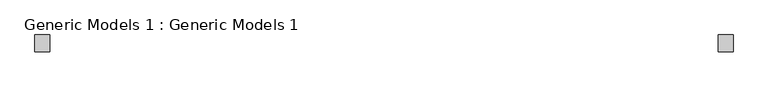
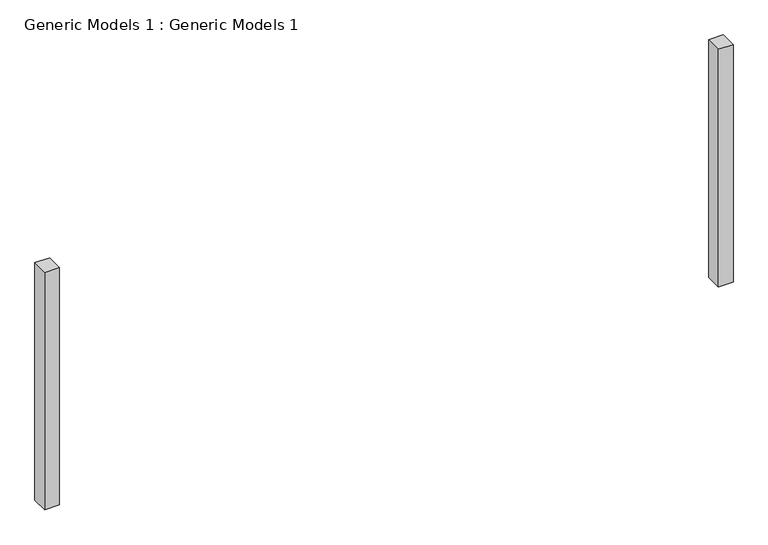
"""IFC4 building model written with IfcOpenShell, lengths in millimetres: proxy geometry, Generic Models 1 : Generic Models 1."""

from ifc_helpers import new_model, si_unit, origin, origin_with_axes, place, context, project, spatial, polyline, outline, extrude, source, transform, mapped, element, save


def generic_models_1_generic_models_1_f4687d58(model_context):
    return source(origin(), model_context, "Body", "SweptSolid", [
        extrude(outline(polyline([(-11120.7803763, 4304.636641), (-11308.7581554, 4304.636641), (-11308.7581554, 4518.2570351), (-11120.7803763, 4518.2570351), (-11120.7803763, 4304.636641)])), origin_with_axes(), (0.0, 0.0, 1.0), 3200.4),
        extrude(outline(polyline([(-2545.7581554, 4518.2570351), (-2545.7581554, 4304.636641), (-2733.7359346, 4304.636641), (-2733.7359346, 4518.2570351), (-2545.7581554, 4518.2570351)])), origin_with_axes(), (0.0, 0.0, 1.0), 3200.4),
    ])


if __name__ == "__main__":
    model = new_model("IFC4")
    model_context = context("Model", 3, world=origin())
    ifc_project = project(units=[si_unit("LENGTHUNIT", "METRE", prefix="MILLI")], contexts=[model_context])
    site = spatial("IfcSite", under=ifc_project)
    building = spatial("IfcBuilding", under=site)
    placement = place(None, origin())
    generic_models_1_generic_models_1_shape = generic_models_1_generic_models_1_f4687d58(model_context)
    element("IfcBuildingElementProxy", 1, Name="Generic Models 1 : Generic Models 1", ObjectType="Generic Models 1 : Generic Models 1", at=placement, inside=building, context=model_context, shape_type="MappedRepresentation", body=[
        mapped(generic_models_1_generic_models_1_shape, transform((0.0, 0.0, 0.0), x_axis=(1.0, 0.0, 0.0), y_axis=(0.0, 1.0, 0.0), z_axis=(0.0, 0.0, 1.0))),
    ])
    save(model, "model.ifc")
